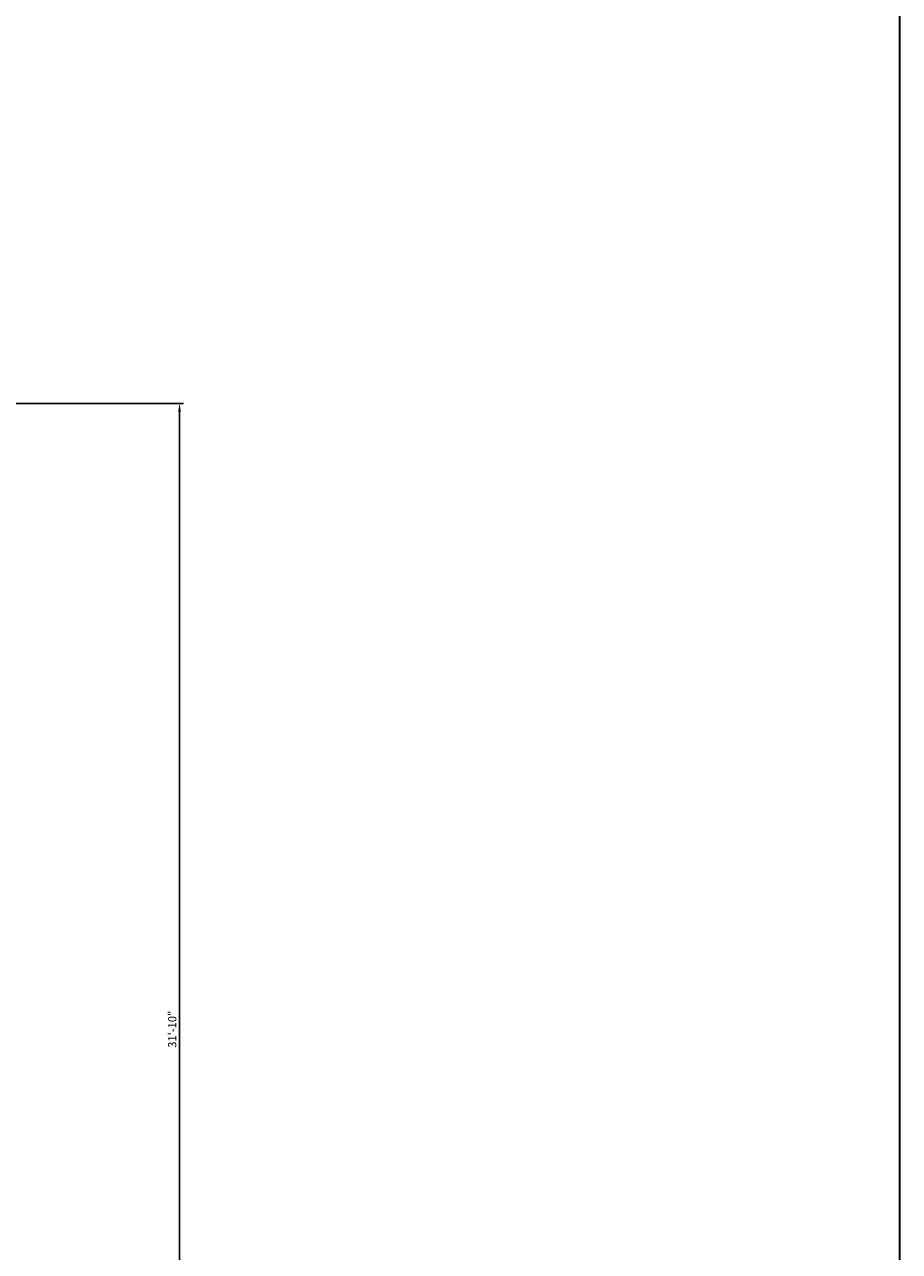
# Model space of a CAD drawing. Units: inches. Extents: x 2020 to 7901, y 1581 to 3943.
# Tile 14 of 17: x 3932 to 4199, y 1955 to 2330. Entities that reach past the tile are written whole.
import ezdxf

# ---------------------------------------------------------------- set-up
doc = ezdxf.new("R2010")
doc.units = ezdxf.units.IN
doc.layers.add('A-ANNO-DIMS', color=2, linetype='Continuous', lineweight=18)
doc.layers.add('A-ANNO-TTLB', color=7, linetype='Continuous', lineweight=35)
doc.styles.get("Standard").update_dxf_attribs({"font": 'arial.ttf'})
doc.dimstyles.new('ISO-25', dxfattribs={"dimtxt": 2.5, "dimasz": 2.5, "dimexe": 1.25, "dimexo": 0.625, "dimtad": 1, "dimdec": 1, "dimlunit": 3, "dimtxsty": 'Standard', "dimcen": 2.5, "dimadec": 0, "dimazin": 0, "dimtfac": 1, "dimtdec": 1, "dimtmove": 0, "dimatfit": 3, "dimfxl": 1, "dimarcsym": 0})

# ---------------------------------------------------------------- blocks, each defined once
blk = doc.blocks.new('*D61')
at = {"layer": 'A-ANNO-DIMS', "color": 0, "lineweight": -2, "transparency": 16777216}
for p, q in [((3868.55, 2214.06), (3980.6, 2214.06)), ((3979.35, 2211.56), (3979.35, 1834.56)), ((3868.55, 1832.06), (3980.6, 1832.06))]:
    blk.add_line(p, q, dxfattribs=at)
at = {"layer": 'A-ANNO-DIMS', "color": 0, "transparency": 16777216}
for points in [[(3978.93, 2211.56), (3979.77, 2211.56), (3979.35, 2214.06)], [(3978.93, 1834.56), (3979.77, 1834.56), (3979.35, 1832.06)]]:
    blk.add_solid(points, dxfattribs=at)
at = {"layer": 'DEFPOINTS', "color": 0, "transparency": 16777216}
for p in [(3867.93, 2214.06), (3867.93, 1832.06), (3979.35, 1832.06)]:
    blk.add_point(p, dxfattribs=at)
at = {"layer": 'A-ANNO-DIMS', "color": 0, "transparency": 16777216, "insert": (3977.45, 2023.06), "char_height": 2.5, "attachment_point": 5, "rotation": 90}
blk.add_mtext('31\'-10"', dxfattribs=at)

msp = doc.modelspace()

# ---------------------------------------------------------------- linework, layer by layer
at = {"layer": 'A-ANNO-TTLB'}
msp.add_lwpolyline([(2019.8, 3067.25), (4199.03, 3067.25), (4199.03, 1580.73), (2019.8, 1580.73)], close=True, dxfattribs=at)

# ---------------------------------------------------------------- dimensions: what is measured, and where the dimension line sits
at = {"layer": 'A-ANNO-DIMS'}
dim = msp.add_linear_dim(base=(3979.35, 1832.06), p1=(3867.93, 2214.06), p2=(3867.93, 1832.06), angle=90, dimstyle='ISO-25', override={"dimdec": 1, "dimlfac": 1, "dimrnd": 0, "dimzin": 1, "dimdsep": 46, "dimlunit": 4, "dimfrac": 2}, dxfattribs=at)
dim.commit()
dim.dimension.update_dxf_attribs({"geometry": '*D61', "text_midpoint": (3977.45, 2023.06)})

doc.saveas('drawing.dxf')
